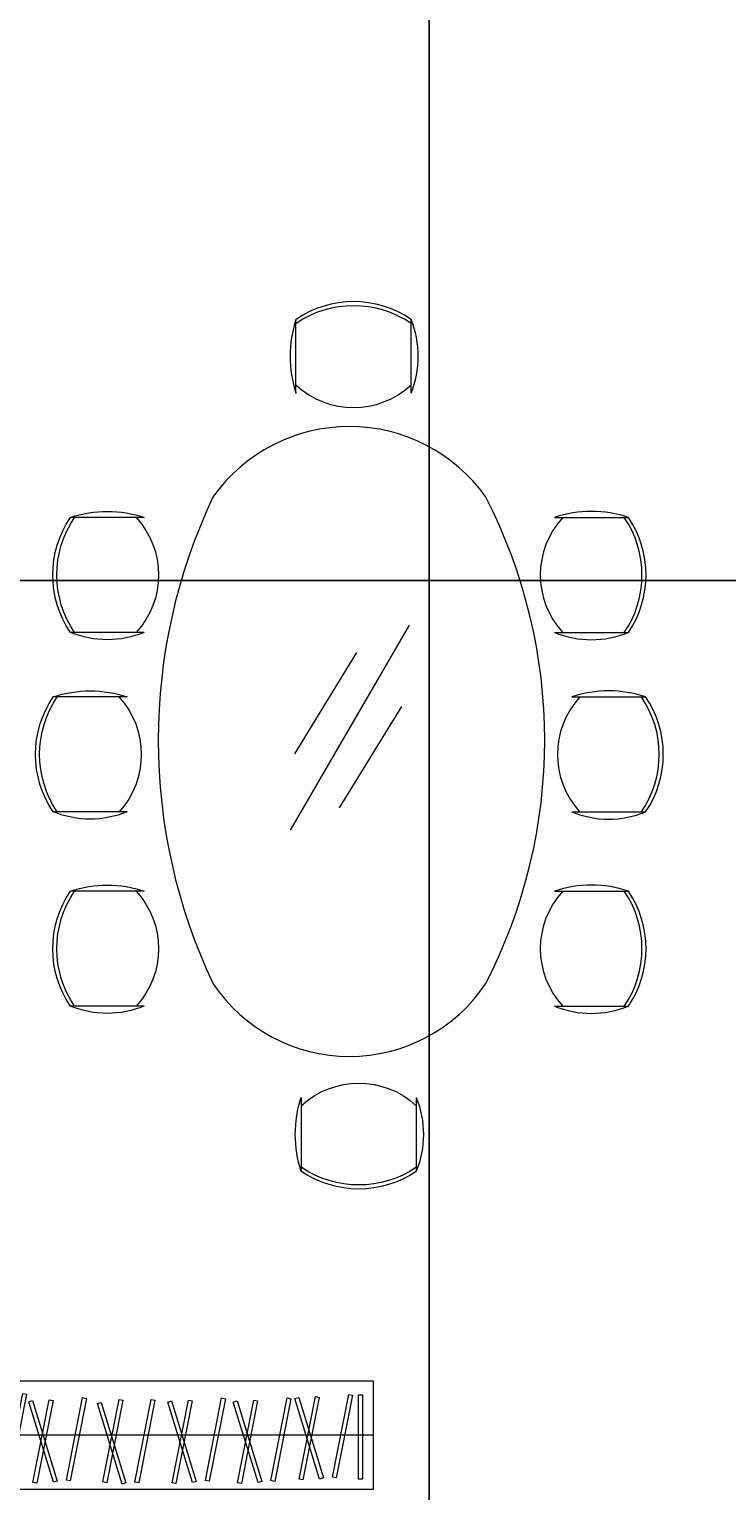
# Model space of a CAD drawing. Units: inches. Extents: x -61 to 1599, y -1316 to 257.
# Tile 21 of 204: x 259 to 365, y -1011 to -790. Entities that reach past the tile are written whole.
import ezdxf

# ---------------------------------------------------------------- set-up
doc = ezdxf.new("R2010")
doc.units = ezdxf.units.IN
doc.header["$MEASUREMENT"] = 0
for name, color, linetype, lineweight in [('A-ANNO-DIMS', 2, 'Continuous', 18), ('A-FLOR-CASE', 8, 'Continuous', 18), ('FURNITURE', 83, 'Continuous', 18)]:
    doc.layers.add(name, color=color, linetype=linetype, lineweight=lineweight)
doc.styles.get("Standard").update_dxf_attribs({"font": 'arial.ttf'})
doc.dimstyles.get("Standard").update_dxf_attribs({"dimtxt": 0.18, "dimasz": 0.18, "dimexe": 0.18, "dimexo": 0.0625, "dimgap": 0.09, "dimtad": 0, "dimtih": 1, "dimtoh": 1, "dimdec": 0, "dimzin": 0, "dimdsep": 46, "dimlunit": 3, "dimtxsty": 'Standard', "dimcen": 0.09, "dimadec": 0, "dimazin": 0, "dimtfac": 1, "dimtdec": 0, "dimtofl": 0, "dimtmove": 0, "dimatfit": 3, "dimfxl": 1, "dimtolj": 1, "dimtzin": 0, "dimarcsym": 0})

# ---------------------------------------------------------------- blocks, each defined once
blk = doc.blocks.new('DINING-TABLE-OVAL')
for p, q in [((20.06, 34.26), (38.12, 65.35)), ((20.69, 45.86), (30.12, 61.18)), ((27.51, 37.68), (36.94, 53.01))]:
    blk.add_line(p, q)
for centre, radius, start, end in [((28.99, 70.07), 25.36, 35.5172, 144.4828), ((85.79, 47.89), 85.79, 154.5151, 205.4849), ((-21.85, 47.89), 80.45, 332.689, 27.311), ((28.99, 24.89), 24.89, 213.9753, 326.0247)]:
    blk.add_arc(centre, radius, start, end)
blk = doc.blocks.new('DINING-CHAIR')
for p, q in [((0.9, 2.16), (0.9, 13.35)), ((18.35, 2.16), (18.35, 13.35))]:
    blk.add_line(p, q)
for centre, radius, start, end in [((9.63, 0.52), 15.52, 55.8098, 124.1902), ((17.78, 7.76), 17.78, 161.6455, 198.3545), ((9.63, -0.1), 15.52, 55.8098, 124.1902), ((4.51, 7.76), 14.92, 337.9646, 22.0354), ((9.63, 12.87), 12.87, 227.332, 312.668)]:
    blk.add_arc(centre, radius, start, end)
blk = doc.blocks.new('WARDROBE-HANGING-2')
blk.add_line((55.7, 8.23), (0, 8.23))
for points in [[(55.7, 16.46), (55.7, 0), (0, 0), (0, 16.46)], [(0.12, 2.03), (2.58, 14.54), (3.16, 14.43), (0.7, 1.92)], [(7.24, 1.1), (3.5, 13.29), (4.06, 13.46), (7.8, 1.28)], [(4.13, 1.08), (6.59, 13.59), (7.17, 13.48), (4.71, 0.97)], [(9.19, 1.4), (11.65, 13.91), (12.23, 13.8), (9.77, 1.29)], [(14.73, 1.14), (17.19, 13.65), (17.77, 13.54), (15.31, 1.03)], [(19.59, 1.12), (22.05, 13.62), (22.63, 13.51), (20.17, 1)], [(28.34, 1.05), (24.59, 13.24), (25.16, 13.41), (28.9, 1.22)], [(25.23, 1.03), (27.69, 13.54), (28.27, 13.43), (25.81, 0.92)], [(30.28, 1.35), (32.74, 13.86), (33.32, 13.75), (30.86, 1.24)], [(38.26, 1.05), (34.51, 13.23), (35.08, 13.41), (38.82, 1.22)], [(35.15, 1.03), (37.61, 13.54), (38.19, 13.42), (35.73, 0.92)], [(40.2, 1.35), (42.66, 13.86), (43.24, 13.74), (40.78, 1.23)], [(47.6, 1.58), (43.86, 13.76), (44.42, 13.94), (48.16, 1.75)], [(44.49, 1.56), (46.95, 14.07), (47.53, 13.95), (45.07, 1.45)], [(49.55, 1.88), (52.01, 14.39), (52.59, 14.27), (50.13, 1.77)], [(54.1, 14.33), (54.1, 1.58), (53.51, 1.58), (53.51, 14.33)], [(17.64, 0.82), (13.9, 13), (14.46, 13.18), (18.2, 0.99)]]:
    blk.add_lwpolyline(points, close=True)
blk = doc.blocks.new('*D687')
at = {"layer": 'A-ANNO-DIMS', "color": 0, "lineweight": -2, "transparency": 16777216}
for p, q in [((289.42, 181.68), (-61.08, 181.68)), ((-60.9, 181.5), (-60.9, -528.95)), ((-60.9, -1239.76), (-60.9, -529.32)), ((319.64, -1239.94), (-61.08, -1239.94))]:
    blk.add_line(p, q, dxfattribs=at)
at = {"layer": 'A-ANNO-DIMS', "color": 0, "transparency": 16777216}
for points in [[(-60.93, 181.5), (-60.87, 181.5), (-60.9, 181.68)], [(-60.93, -1239.76), (-60.87, -1239.76), (-60.9, -1239.94)]]:
    blk.add_solid(points, dxfattribs=at)
at = {"layer": 'DEFPOINTS', "color": 0, "transparency": 16777216}
for p in [(289.48, 181.68), (-60.9, -1239.94), (319.7, -1239.94)]:
    blk.add_point(p, dxfattribs=at)
at = {"layer": 'A-ANNO-DIMS', "color": 0, "transparency": 16777216, "insert": (-60.9, -529.13), "char_height": 0.18, "attachment_point": 5}
blk.add_mtext('\\A1;1421.6', dxfattribs=at)
blk = doc.blocks.new('*D696')
at = {"layer": 'A-ANNO-DIMS', "color": 0, "lineweight": -2, "transparency": 16777216}
for p, q in [((690.64, -873.17), (-61.08, -873.17)), ((-60.9, -873.35), (-60.9, -1025.8)), ((-60.9, -1178.61), (-60.9, -1026.16)), ((690.64, -1178.79), (-61.08, -1178.79))]:
    blk.add_line(p, q, dxfattribs=at)
at = {"layer": 'A-ANNO-DIMS', "color": 0, "transparency": 16777216}
for points in [[(-60.93, -873.35), (-60.87, -873.35), (-60.9, -873.17)], [(-60.93, -1178.61), (-60.87, -1178.61), (-60.9, -1178.79)]]:
    blk.add_solid(points, dxfattribs=at)
at = {"layer": 'DEFPOINTS', "color": 0, "transparency": 16777216}
for p in [(-60.9, -873.17), (690.7, -873.17), (690.7, -1178.79)]:
    blk.add_point(p, dxfattribs=at)
at = {"layer": 'A-ANNO-DIMS', "color": 0, "transparency": 16777216, "insert": (-60.9, -1025.98), "char_height": 0.18, "attachment_point": 5}
blk.add_mtext('\\A1;305.6', dxfattribs=at)
blk = doc.blocks.new('*D710')
at = {"layer": 'A-ANNO-DIMS', "color": 0, "lineweight": -2, "transparency": 16777216}
for p, q in [((319.7, -465.39), (319.7, -1315.72)), ((403.7, -465.39), (403.7, -1315.72)), ((319.88, -1315.54), (361.48, -1315.54)), ((403.52, -1315.54), (361.92, -1315.54))]:
    blk.add_line(p, q, dxfattribs=at)
at = {"layer": 'A-ANNO-DIMS', "color": 0, "transparency": 16777216}
for points in [[(319.88, -1315.51), (319.88, -1315.57), (319.7, -1315.54)], [(403.52, -1315.51), (403.52, -1315.57), (403.7, -1315.54)]]:
    blk.add_solid(points, dxfattribs=at)
at = {"layer": 'DEFPOINTS', "color": 0, "transparency": 16777216}
for p in [(319.7, -465.32), (403.7, -465.32), (403.7, -1315.54)]:
    blk.add_point(p, dxfattribs=at)
at = {"layer": 'A-ANNO-DIMS', "color": 0, "transparency": 16777216, "insert": (361.7, -1315.54), "char_height": 0.18, "attachment_point": 5}
blk.add_mtext('\\A1;84', dxfattribs=at)

msp = doc.modelspace()

# ---------------------------------------------------------------- block references
at = {"layer": 'A-FLOR-CASE'}
msp.add_blockref('WARDROBE-HANGING-2', (255.5089, -1010.847), dxfattribs=at)
at = {"layer": 'FURNITURE'}
for name, p in [('DINING-CHAIR', (298.622, -846.9457)), ('DINING-TABLE-OVAL', (278.634, -945.2477))]:
    msp.add_blockref(name, p, dxfattribs=at)
at = {"layer": 'FURNITURE', "extrusion": (0, 0, -1), "zscale": -1}
for p, rotation in [((-278.681, -862.6846), 269.9999999999998), ((-276.0669, -889.8661), 269.9999999999992), ((-278.681, -919.2915), 270.0000000000001), ((-299.4166, -949.2994), 180)]:
    msp.add_blockref('DINING-CHAIR', p, dxfattribs=dict(at, rotation=rotation))
at = {"layer": 'FURNITURE'}
for p, rotation in [((336.562, -862.6846), 269.9999999999984), ((339.1761, -889.8661), 269.9999999999996), ((336.562, -919.2915), 269.9999999999984)]:
    msp.add_blockref('DINING-CHAIR', p, dxfattribs=dict(at, rotation=rotation))

# ---------------------------------------------------------------- dimensions: what is measured, and where the dimension line sits
at = {"layer": 'A-ANNO-DIMS'}
for base, p1, p2, picture, middle in [((-60.8972, -1239.9446), (289.4807, 181.6771), (319.7028, -1239.9446), '*D687', (-60.8972, -529.1337)), ((-60.8972, -873.169), (690.7028, -1178.7933), (690.7028, -873.169), '*D696', (-60.8972, -1025.9812))]:
    dim = msp.add_linear_dim(base=base, p1=p1, p2=p2, angle=90, dimstyle='Standard', override={"dimdec": 1, "dimlfac": 1, "dimrnd": 0, "dimzin": 0, "dimdsep": 46, "dimlunit": 2}, dxfattribs=at)
    dim.commit()
    dim.dimension.update_dxf_attribs({"geometry": picture, "text_midpoint": middle})
dim = msp.add_linear_dim(base=(403.7028, -1315.5446), p1=(319.7028, -465.3229), p2=(403.7028, -465.3229), dimstyle='Standard', override={"dimdec": 0, "dimlfac": 1, "dimrnd": 0, "dimzin": 0, "dimdsep": 46, "dimlunit": 2}, dxfattribs=at)
dim.commit()
dim.dimension.update_dxf_attribs({"geometry": '*D710', "text_midpoint": (361.7028, -1315.5446)})

doc.saveas('drawing.dxf')
